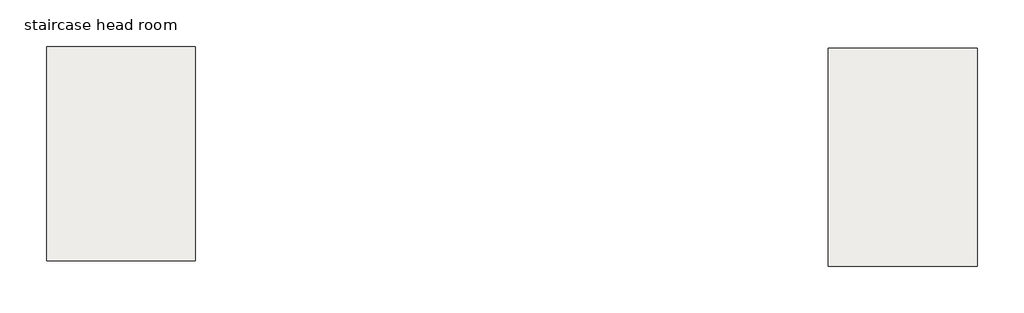
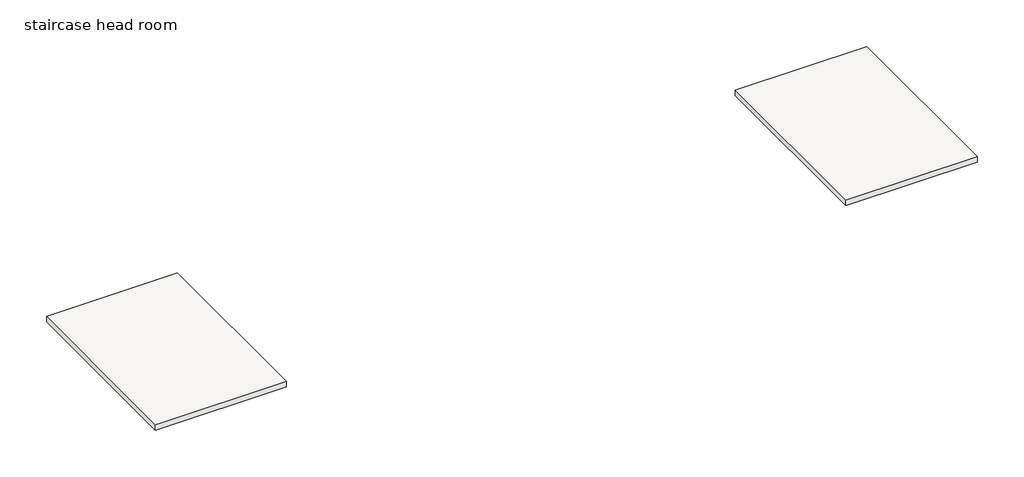
# One storey: 2 slabs.
"""IFC4 building model written with IfcOpenShell, lengths in millimetres."""

from ifc_helpers import new_model, si_unit, frame, origin, place, context, project, spatial, polyline, outline, extrude, element, save

model = new_model("IFC4")

# Units and contexts
model_context = context("Model", 3, world=origin())
ifc_project = project(units=[si_unit("LENGTHUNIT", "METRE", prefix="MILLI")], contexts=[model_context])

# Site, building, storey
site = spatial("IfcSite", under=ifc_project)
building = spatial("IfcBuilding", under=site)
storey = spatial("IfcBuildingStorey", under=building, Name="staircase head room", Elevation=9753.6)

# Slabs
placement = place(None, origin())
element("IfcSlab", 1, at=placement, inside=storey, context=model_context, shape_type="SweptSolid", body=[
    extrude(outline(polyline([(-1962.2993763, -274.6064015), (-1962.2993763, -5176.8064015), (-5365.8993763, -5176.8064015), (-5365.8993763, -274.6064015), (-1962.2993763, -274.6064015)])), frame((0.0, 0.0, 9601.2), z_axis=(0.0, 0.0, 1.0), x_axis=(1.0, 0.0, 0.0)), (0.0, 0.0, 1.0), 152.4),
])
element("IfcSlab", 2, at=placement, inside=storey, context=model_context, shape_type="SweptSolid", body=[
    extrude(outline(polyline([(15925.6506237, -319.0564015), (15925.6506237, -5303.8064015), (12508.6761273, -5303.8064015), (12508.6761273, -319.0564015), (15925.6506237, -319.0564015)])), frame((0.0, 0.0, 9601.2), z_axis=(0.0, 0.0, 1.0), x_axis=(1.0, 0.0, 0.0)), (0.0, 0.0, 1.0), 152.4),
])

save(model, "model.ifc")

# Revit data of these elements
# Type
#   Assembly Code = "B1010"
#   Function = 0
#   Layers, outside or top first: 0' - 6" "Concrete, Cast-in-Place gray" (function 1)
# Elements 1, 2 (IfcSlab)
#   Height Offset From Level = 0' - 0"
#   Phase Created = New Construction
#   Materials on its faces: "Concrete, Cast-in-Place gray"
# Materials
#   "Concrete, Cast-in-Place gray": class "Concrete", colour RGB 192 192 192, transparency 0, Description = "Cast-in-place concrete", Cost = 0
